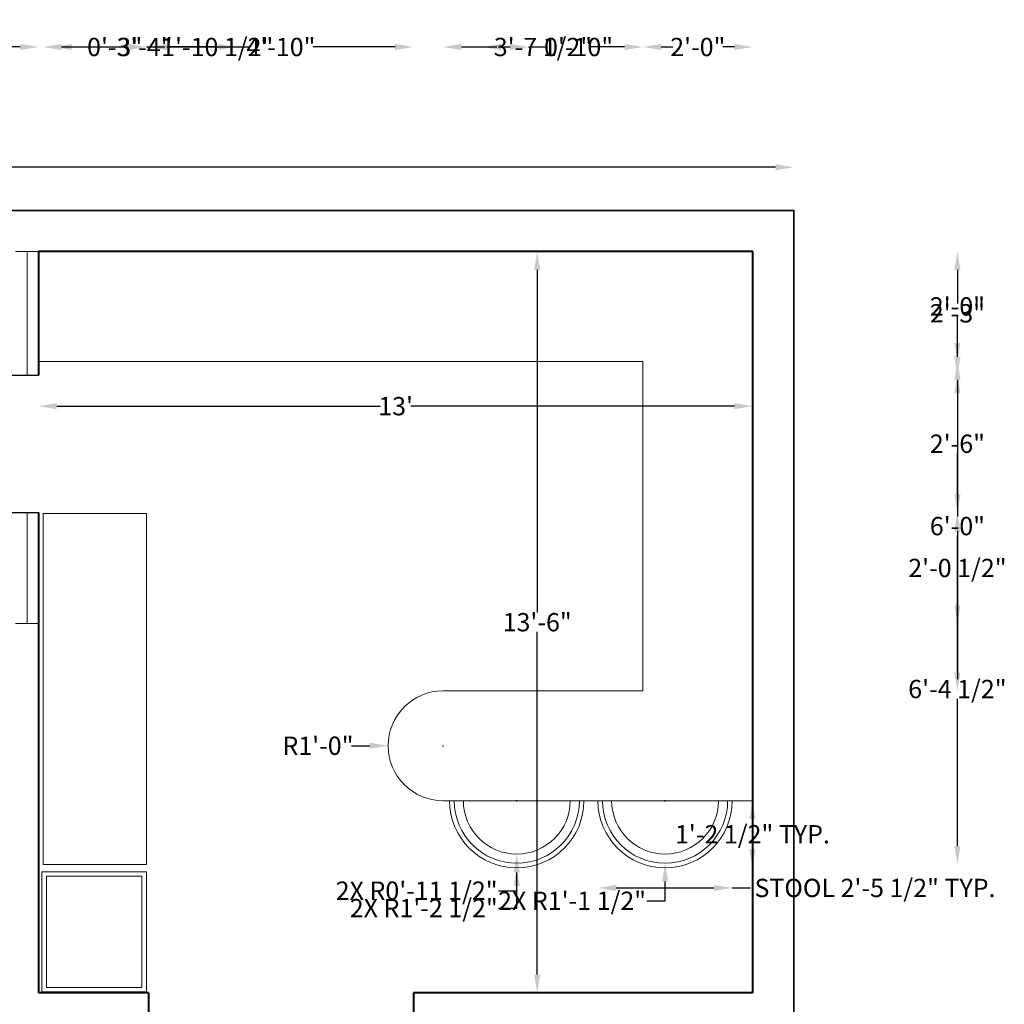
# Model space of a CAD drawing. Units: inches. Extents: x -46 to 447, y -42 to 702.
# Tile 7 of 7: x 227 to 442, y 487 to 702. Entities that reach past the tile are written whole.
import ezdxf

# ---------------------------------------------------------------- set-up
doc = ezdxf.new("R2010")
doc.units = ezdxf.units.IN
doc.header["$PDMODE"] = 3
for name, color, linetype, lineweight in [('A-ANNO-DIMS', 2, 'Continuous', 13), ('A-DOOR', 3, 'Continuous', 25), ('A-FLOR-CASE', 32, 'Continuous', 18), ('A-FURN', 8, 'Continuous', 18), ('A-GLAZ', 4, 'Continuous', 18), ('A-WALL', 7, 'Continuous', 40), ('L-WALL', 7, 'Continuous', 35)]:
    doc.layers.add(name, color=color, linetype=linetype, lineweight=lineweight)
doc.styles.get("Standard").update_dxf_attribs({"font": 'arial.ttf'})
doc.dimstyles.get("Standard").update_dxf_attribs({"dimtxt": 4, "dimasz": 4, "dimexe": 0.18, "dimexo": 0.0625, "dimgap": 0.09, "dimtad": 0, "dimtih": 1, "dimtoh": 1, "dimdec": 0, "dimzin": 0, "dimdsep": 46, "dimlunit": 3, "dimtxsty": 'Standard', "dimcen": 0.09, "dimse1": 1, "dimse2": 1, "dimadec": 0, "dimazin": 0, "dimtfac": 1, "dimtdec": 0, "dimtofl": 0, "dimtmove": 0, "dimatfit": 3, "dimfxl": 1, "dimtolj": 1, "dimtzin": 0, "dimarcsym": 0})

# ---------------------------------------------------------------- blocks, each defined once
blk = doc.blocks.new('*U3')
for p, q in [((-30, 0), (-30, -6)), ((0, 0), (0, -6))]:
    blk.add_line(p, q)
blk.add_lwpolyline([(0, 0), (0, 30), (-1.75, 30), (-1.75, 0)], close=True)
blk.add_arc((0, 0), 30, 90, 180)
blk = doc.blocks.new('*D49')
at = {"layer": 'A-ANNO-DIMS', "color": 0, "lineweight": -2, "transparency": 16777216}
for p, q in [((4, 669.42), (194.52, 669.42)), ((392, 669.42), (201.48, 669.42))]:
    blk.add_line(p, q, dxfattribs=at)
at = {"layer": 'A-ANNO-DIMS', "color": 0, "transparency": 16777216}
for points in [[(4, 670.09), (4, 668.76), (0, 669.42)], [(392, 670.09), (392, 668.76), (396, 669.42)]]:
    blk.add_solid(points, dxfattribs=at)
at = {"layer": 'Defpoints', "color": 0, "transparency": 16777216}
for p in [(396, 669.42), (0, 660), (396, 660)]:
    blk.add_point(p, dxfattribs=at)
at = {"layer": 'A-ANNO-DIMS', "color": 0, "transparency": 16777216, "insert": (198, 669.42), "char_height": 4, "attachment_point": 5}
blk.add_mtext("\\A1;33'", dxfattribs=at)
blk = doc.blocks.new('*D71')
at = {"layer": 'A-ANNO-DIMS', "color": 0, "lineweight": -2, "transparency": 16777216}
for p, q in [((235, 617.21), (305.7, 617.21)), ((383, 617.21), (312.3, 617.21))]:
    blk.add_line(p, q, dxfattribs=at)
at = {"layer": 'A-ANNO-DIMS', "color": 0, "transparency": 16777216}
for points in [[(235, 617.88), (235, 616.55), (231, 617.21)], [(383, 617.88), (383, 616.55), (387, 617.21)]]:
    blk.add_solid(points, dxfattribs=at)
at = {"layer": 'Defpoints', "color": 0, "transparency": 16777216}
for p in [(231, 651), (387, 651), (231, 617.21)]:
    blk.add_point(p, dxfattribs=at)
at = {"layer": 'A-ANNO-DIMS', "color": 0, "transparency": 16777216, "insert": (309, 617.21), "char_height": 4, "attachment_point": 5}
blk.add_mtext("\\A1;13'", dxfattribs=at)
blk = doc.blocks.new('*D72')
at = {"layer": 'A-ANNO-DIMS', "color": 0, "lineweight": -2, "transparency": 16777216}
for p, q in [((339.92, 647), (339.92, 572.13)), ((339.92, 493), (339.92, 567.87))]:
    blk.add_line(p, q, dxfattribs=at)
at = {"layer": 'A-ANNO-DIMS', "color": 0, "transparency": 16777216}
for points in [[(339.26, 647), (340.59, 647), (339.92, 651)], [(339.26, 493), (340.59, 493), (339.92, 489)]]:
    blk.add_solid(points, dxfattribs=at)
at = {"layer": 'Defpoints', "color": 0, "transparency": 16777216}
for p in [(339.92, 651), (387, 651), (387, 489)]:
    blk.add_point(p, dxfattribs=at)
at = {"layer": 'A-ANNO-DIMS', "color": 0, "transparency": 16777216, "insert": (339.92, 570), "char_height": 4, "attachment_point": 5}
blk.add_mtext('\\A1;13\'-6"', dxfattribs=at)
blk = doc.blocks.new('COUNTER-STOOL')
for radius in [14.67, 13.67, 11.67]:
    blk.add_arc((0, 0), radius, 180, 0)
blk = doc.blocks.new('*D102')
at = {"layer": 'A-ANNO-DIMS', "color": 0, "lineweight": -2, "transparency": 16777216}
for p, q in [((357.18, 511.93), (378.53, 511.93)), ((382.53, 511.93), (386.53, 511.93))]:
    blk.add_line(p, q, dxfattribs=at)
at = {"layer": 'A-ANNO-DIMS', "color": 0, "transparency": 16777216}
for points in [[(357.18, 512.59), (357.18, 511.26), (353.18, 511.93)], [(378.53, 512.59), (378.53, 511.26), (382.53, 511.93)]]:
    blk.add_solid(points, dxfattribs=at)
at = {"layer": 'Defpoints', "color": 0, "transparency": 16777216}
for p in [(353.18, 516.33), (382.53, 516.33), (382.53, 511.93)]:
    blk.add_point(p, dxfattribs=at)
at = {"layer": 'A-ANNO-DIMS', "color": 0, "transparency": 16777216, "insert": (413.7, 511.93), "char_height": 4, "attachment_point": 5}
blk.add_mtext('\\A1;STOOL 2\'-5 1/2" TYP.', dxfattribs=at)
blk = doc.blocks.new('*D103')
at = {"layer": 'A-ANNO-DIMS', "color": 0, "lineweight": -2, "transparency": 16777216}
for p, q in [((386.93, 527), (386.93, 525.82)), ((386.93, 520.33), (386.93, 521.51))]:
    blk.add_line(p, q, dxfattribs=at)
at = {"layer": 'A-ANNO-DIMS', "color": 0, "transparency": 16777216}
for points in [[(386.26, 527), (387.59, 527), (386.93, 531)], [(386.26, 520.33), (387.59, 520.33), (386.93, 516.33)]]:
    blk.add_solid(points, dxfattribs=at)
at = {"layer": 'Defpoints', "color": 0, "transparency": 16777216}
for p in [(382.53, 531), (386.93, 531), (382.53, 516.33)]:
    blk.add_point(p, dxfattribs=at)
at = {"layer": 'A-ANNO-DIMS', "color": 0, "transparency": 16777216, "insert": (386.93, 523.66), "char_height": 4, "attachment_point": 5}
blk.add_mtext('\\A1;1\'-2 1/2" TYP.', dxfattribs=at)
blk = doc.blocks.new('*D116')
at = {"layer": 'A-ANNO-DIMS', "color": 0, "lineweight": -2, "transparency": 16777216}
for p, q in [((367, 695.7), (369.56, 695.7)), ((383, 695.7), (380.44, 695.7))]:
    blk.add_line(p, q, dxfattribs=at)
at = {"layer": 'A-ANNO-DIMS', "color": 0, "transparency": 16777216}
for points in [[(367, 696.37), (367, 695.03), (363, 695.7)], [(383, 696.37), (383, 695.03), (387, 695.7)]]:
    blk.add_solid(points, dxfattribs=at)
at = {"layer": 'Defpoints', "color": 0, "transparency": 16777216}
for p in [(387, 695.7), (387, 651), (363, 627)]:
    blk.add_point(p, dxfattribs=at)
at = {"layer": 'A-ANNO-DIMS', "color": 0, "transparency": 16777216, "insert": (375, 695.7), "char_height": 4, "attachment_point": 5}
blk.add_mtext('\\A1;2\'-0"', dxfattribs=at)
blk = doc.blocks.new('*D117')
at = {"layer": 'A-ANNO-DIMS', "color": 0, "lineweight": -2, "transparency": 16777216}
for p, q in [((259, 695.7), (276.91, 695.7)), ((308.89, 695.7), (290.99, 695.7))]:
    blk.add_line(p, q, dxfattribs=at)
at = {"layer": 'A-ANNO-DIMS', "color": 0, "transparency": 16777216}
for points in [[(259, 696.37), (259, 695.03), (255, 695.7)], [(308.89, 696.37), (308.89, 695.03), (312.89, 695.7)]]:
    blk.add_solid(points, dxfattribs=at)
at = {"layer": 'Defpoints', "color": 0, "transparency": 16777216}
for p in [(312.89, 695.7), (255, 489), (312.89, 489)]:
    blk.add_point(p, dxfattribs=at)
at = {"layer": 'A-ANNO-DIMS', "color": 0, "transparency": 16777216, "insert": (283.95, 695.7), "char_height": 4, "attachment_point": 5}
blk.add_mtext('\\A1;4\'-10"', dxfattribs=at)
blk = doc.blocks.new('*D119')
at = {"layer": 'A-ANNO-DIMS', "color": 0, "lineweight": -2, "transparency": 16777216}
for p, q in [((238.24, 695.7), (248.83, 695.7)), ((270.24, 695.7), (259.64, 695.7))]:
    blk.add_line(p, q, dxfattribs=at)
at = {"layer": 'A-ANNO-DIMS', "color": 0, "transparency": 16777216}
for points in [[(238.24, 696.37), (238.24, 695.03), (234.24, 695.7)], [(270.24, 696.37), (270.24, 695.03), (274.24, 695.7)]]:
    blk.add_solid(points, dxfattribs=at)
at = {"layer": 'Defpoints', "color": 0, "transparency": 16777216}
for p in [(274.24, 695.7), (234.24, 319), (274.24, 319)]:
    blk.add_point(p, dxfattribs=at)
at = {"layer": 'A-ANNO-DIMS', "color": 0, "transparency": 16777216, "insert": (254.24, 695.7), "char_height": 4, "attachment_point": 5}
blk.add_mtext('\\A1;3\'-4"', dxfattribs=at)
blk = doc.blocks.new('*D124')
at = {"layer": 'A-ANNO-DIMS', "color": 0, "lineweight": -2, "transparency": 16777216}
for p, q in [((431.7, 620), (431.7, 611.13)), ((431.7, 598), (431.7, 606.87))]:
    blk.add_line(p, q, dxfattribs=at)
at = {"layer": 'A-ANNO-DIMS', "color": 0, "transparency": 16777216}
for points in [[(431.03, 620), (432.37, 620), (431.7, 624)], [(431.03, 598), (432.37, 598), (431.7, 594)]]:
    blk.add_solid(points, dxfattribs=at)
at = {"layer": 'Defpoints', "color": 0, "transparency": 16777216}
for p in [(231, 624), (431.7, 624), (231, 594)]:
    blk.add_point(p, dxfattribs=at)
at = {"layer": 'A-ANNO-DIMS', "color": 0, "transparency": 16777216, "insert": (431.7, 609), "char_height": 4, "attachment_point": 5}
blk.add_mtext('\\A1;2\'-6"', dxfattribs=at)
blk = doc.blocks.new('*D134')
at = {"layer": 'A-ANNO-DIMS', "color": 0, "lineweight": -2, "transparency": 16777216}
for p, q in [((431.7, 623), (431.7, 593.13)), ((431.7, 559), (431.7, 588.87))]:
    blk.add_line(p, q, dxfattribs=at)
at = {"layer": 'A-ANNO-DIMS', "color": 0, "transparency": 16777216}
for points in [[(431.03, 623), (432.37, 623), (431.7, 627)], [(431.03, 559), (432.37, 559), (431.7, 555)]]:
    blk.add_solid(points, dxfattribs=at)
at = {"layer": 'Defpoints', "color": 0, "transparency": 16777216}
for p in [(363, 627), (363, 555), (431.7, 555)]:
    blk.add_point(p, dxfattribs=at)
at = {"layer": 'A-ANNO-DIMS', "color": 0, "transparency": 16777216, "insert": (431.7, 591), "char_height": 4, "attachment_point": 5}
blk.add_mtext('\\A1;6\'-0"', dxfattribs=at)
blk = doc.blocks.new('*D135')
at = {"layer": 'A-ANNO-DIMS', "color": 0, "lineweight": -2, "transparency": 16777216}
for p, q in [((323.36, 695.7), (331.11, 695.7)), ((359, 695.7), (351.25, 695.7))]:
    blk.add_line(p, q, dxfattribs=at)
at = {"layer": 'A-ANNO-DIMS', "color": 0, "transparency": 16777216}
for points in [[(323.36, 696.37), (323.36, 695.03), (319.36, 695.7)], [(359, 696.37), (359, 695.03), (363, 695.7)]]:
    blk.add_solid(points, dxfattribs=at)
at = {"layer": 'Defpoints', "color": 0, "transparency": 16777216}
for p in [(363, 695.7), (319.36, 555), (363, 555)]:
    blk.add_point(p, dxfattribs=at)
at = {"layer": 'A-ANNO-DIMS', "color": 0, "transparency": 16777216, "insert": (341.18, 695.7), "char_height": 4, "attachment_point": 5}
blk.add_mtext('\\A1;3\'-7 1/2"', dxfattribs=at)
blk = doc.blocks.new('*D136')
at = {"layer": 'A-ANNO-DIMS', "color": 0, "lineweight": -2, "transparency": 16777216}
for p, q in [((431.7, 647), (431.7, 641.13)), ((431.7, 631), (431.7, 636.87))]:
    blk.add_line(p, q, dxfattribs=at)
at = {"layer": 'A-ANNO-DIMS', "color": 0, "transparency": 16777216}
for points in [[(431.03, 647), (432.37, 647), (431.7, 651)], [(431.03, 631), (432.37, 631), (431.7, 627)]]:
    blk.add_solid(points, dxfattribs=at)
at = {"layer": 'Defpoints', "color": 0, "transparency": 16777216}
for p in [(387, 651), (431.7, 651), (363, 627)]:
    blk.add_point(p, dxfattribs=at)
at = {"layer": 'A-ANNO-DIMS', "color": 0, "transparency": 16777216, "insert": (431.7, 639), "char_height": 4, "attachment_point": 5}
blk.add_mtext('\\A1;2\'-0"', dxfattribs=at)
blk = doc.blocks.new('*D139')
at = {"layer": 'A-ANNO-DIMS', "color": 0, "lineweight": -2, "transparency": 16777216}
for p, q in [((431.7, 590), (431.7, 584.01)), ((431.7, 573.71), (431.7, 579.7))]:
    blk.add_line(p, q, dxfattribs=at)
at = {"layer": 'A-ANNO-DIMS', "color": 0, "transparency": 16777216}
for points in [[(431.03, 590), (432.37, 590), (431.7, 594)], [(431.03, 573.71), (432.37, 573.71), (431.7, 569.71)]]:
    blk.add_solid(points, dxfattribs=at)
at = {"layer": 'Defpoints', "color": 0, "transparency": 16777216}
for p in [(226, 594), (431.7, 594), (226, 569.71)]:
    blk.add_point(p, dxfattribs=at)
at = {"layer": 'A-ANNO-DIMS', "color": 0, "transparency": 16777216, "insert": (431.7, 581.85), "char_height": 4, "attachment_point": 5}
blk.add_mtext('\\A1;2\'-0 1/2"', dxfattribs=at)
blk = doc.blocks.new('*D142')
at = {"layer": 'A-ANNO-DIMS', "color": 0, "lineweight": -2, "transparency": 16777216}
for p, q in [((431.7, 647), (431.7, 639.63)), ((431.7, 628), (431.7, 635.37))]:
    blk.add_line(p, q, dxfattribs=at)
at = {"layer": 'A-ANNO-DIMS', "color": 0, "transparency": 16777216}
for points in [[(431.03, 647), (432.37, 647), (431.7, 651)], [(431.03, 628), (432.37, 628), (431.7, 624)]]:
    blk.add_solid(points, dxfattribs=at)
at = {"layer": 'Defpoints', "color": 0, "transparency": 16777216}
for p in [(231, 651), (431.7, 651), (231, 624)]:
    blk.add_point(p, dxfattribs=at)
at = {"layer": 'A-ANNO-DIMS', "color": 0, "transparency": 16777216, "insert": (431.7, 637.5), "char_height": 4, "attachment_point": 5}
blk.add_mtext('\\A1;2\'-3"', dxfattribs=at)
blk = doc.blocks.new('*D148')
at = {"layer": 'A-ANNO-DIMS', "color": 0, "lineweight": -2, "transparency": 16777216}
for p, q in [((227, 695.7), (223, 695.7)), ((238.24, 695.7), (242.24, 695.7))]:
    blk.add_line(p, q, dxfattribs=at)
at = {"layer": 'A-ANNO-DIMS', "color": 0, "transparency": 16777216}
for points in [[(227, 696.37), (227, 695.03), (231, 695.7)], [(238.24, 696.37), (238.24, 695.03), (234.24, 695.7)]]:
    blk.add_solid(points, dxfattribs=at)
at = {"layer": 'Defpoints', "color": 0, "transparency": 16777216}
for p in [(234.24, 695.7), (231, 319), (234.24, 319)]:
    blk.add_point(p, dxfattribs=at)
at = {"layer": 'A-ANNO-DIMS', "color": 0, "transparency": 16777216, "insert": (247.64, 695.7), "char_height": 4, "attachment_point": 5}
blk.add_mtext('\\A1;0\'-3"', dxfattribs=at)
blk = doc.blocks.new('*D149')
at = {"layer": 'A-ANNO-DIMS', "color": 0, "lineweight": -2, "transparency": 16777216}
for p, q in [((332, 695.7), (334, 695.7)), ((338, 695.7), (342, 695.7))]:
    blk.add_line(p, q, dxfattribs=at)
at = {"layer": 'A-ANNO-DIMS', "color": 0, "transparency": 16777216}
for points in [[(332, 696.37), (332, 695.03), (328, 695.7)], [(334, 696.37), (334, 695.03), (338, 695.7)]]:
    blk.add_solid(points, dxfattribs=at)
at = {"layer": 'Defpoints', "color": 0, "transparency": 16777216}
for p in [(338, 695.7), (328, 445), (338, 445)]:
    blk.add_point(p, dxfattribs=at)
at = {"layer": 'A-ANNO-DIMS', "color": 0, "transparency": 16777216, "insert": (348.96, 695.7), "char_height": 4, "attachment_point": 5}
blk.add_mtext('\\A1;0\'-10"', dxfattribs=at)
blk = doc.blocks.new('*D151')
at = {"layer": 'A-ANNO-DIMS', "color": 0, "lineweight": -2, "transparency": 16777216}
for p, q in [((236.01, 695.7), (250.6, 695.7)), ((254.6, 695.7), (258.6, 695.7))]:
    blk.add_line(p, q, dxfattribs=at)
at = {"layer": 'A-ANNO-DIMS', "color": 0, "transparency": 16777216}
for points in [[(236.01, 696.37), (236.01, 695.03), (232.01, 695.7)], [(250.6, 696.37), (250.6, 695.03), (254.6, 695.7)]]:
    blk.add_solid(points, dxfattribs=at)
at = {"layer": 'Defpoints', "color": 0, "transparency": 16777216}
for p in [(254.6, 695.7), (232.01, 593.76), (254.6, 593.76)]:
    blk.add_point(p, dxfattribs=at)
at = {"layer": 'A-ANNO-DIMS', "color": 0, "transparency": 16777216, "insert": (270.04, 695.7), "char_height": 4, "attachment_point": 5}
blk.add_mtext('\\A1;1\'-10 1/2"', dxfattribs=at)
blk = doc.blocks.new('*D152')
at = {"layer": 'A-ANNO-DIMS', "color": 0, "lineweight": -2, "transparency": 16777216}
for p, q in [((431.7, 589.76), (431.7, 557.56)), ((431.7, 521.03), (431.7, 553.24))]:
    blk.add_line(p, q, dxfattribs=at)
at = {"layer": 'A-ANNO-DIMS', "color": 0, "transparency": 16777216}
for points in [[(431.03, 589.76), (432.37, 589.76), (431.7, 593.76)], [(431.03, 521.03), (432.37, 521.03), (431.7, 517.03)]]:
    blk.add_solid(points, dxfattribs=at)
at = {"layer": 'Defpoints', "color": 0, "transparency": 16777216}
for p in [(254.6, 593.76), (254.6, 517.03), (431.7, 517.03)]:
    blk.add_point(p, dxfattribs=at)
at = {"layer": 'A-ANNO-DIMS', "color": 0, "transparency": 16777216, "insert": (431.7, 555.4), "char_height": 4, "attachment_point": 5}
blk.add_mtext('\\A1;6\'-4 1/2"', dxfattribs=at)
blk = doc.blocks.new('*D155')
at = {"layer": 'A-ANNO-DIMS', "color": 0, "lineweight": -2, "transparency": 16777216}
for p, q in [((299.36, 543), (303.36, 543)), ((319.27, 543), (319.45, 543)), ((319.36, 542.91), (319.36, 543.09))]:
    blk.add_line(p, q, dxfattribs=at)
at = {"layer": 'A-ANNO-DIMS', "color": 0, "transparency": 16777216}
blk.add_solid([(303.36, 543.67), (303.36, 542.33), (307.36, 543)], dxfattribs=at)
at = {"layer": 'Defpoints', "color": 0, "transparency": 16777216}
for p in [(307.36, 543), (319.36, 543)]:
    blk.add_point(p, dxfattribs=at)
at = {"layer": 'A-ANNO-DIMS', "color": 0, "transparency": 16777216, "insert": (292.04, 543), "char_height": 4, "attachment_point": 5}
blk.add_mtext('\\A1;R1\'-0"', dxfattribs=at)
blk = doc.blocks.new('*D156')
at = {"layer": 'A-ANNO-DIMS', "color": 0, "lineweight": -2, "transparency": 16777216}
for p, q in [((335.37, 531), (335.55, 531)), ((335.46, 530.91), (335.46, 531.09)), ((335.46, 507.52), (335.46, 512.33)), ((331.46, 507.52), (335.46, 507.52))]:
    blk.add_line(p, q, dxfattribs=at)
at = {"layer": 'A-ANNO-DIMS', "color": 0, "transparency": 16777216}
blk.add_solid([(334.79, 512.33), (336.13, 512.33), (335.46, 516.33)], dxfattribs=at)
at = {"layer": 'Defpoints', "color": 0, "transparency": 16777216}
for p in [(335.46, 531), (335.46, 516.33)]:
    blk.add_point(p, dxfattribs=at)
at = {"layer": 'A-ANNO-DIMS', "color": 0, "transparency": 16777216, "insert": (315.15, 507.52), "char_height": 4, "attachment_point": 5}
blk.add_mtext('\\A1;2X R1\'-2 1/2"', dxfattribs=at)
blk = doc.blocks.new('*D157')
at = {"layer": 'A-ANNO-DIMS', "color": 0, "lineweight": -2, "transparency": 16777216}
for p, q in [((367.76, 531), (367.94, 531)), ((367.85, 530.91), (367.85, 531.09)), ((367.85, 509.12), (367.85, 513.33)), ((363.85, 509.12), (367.85, 509.12))]:
    blk.add_line(p, q, dxfattribs=at)
at = {"layer": 'A-ANNO-DIMS', "color": 0, "transparency": 16777216}
blk.add_solid([(367.19, 513.33), (368.52, 513.33), (367.85, 517.33)], dxfattribs=at)
at = {"layer": 'Defpoints', "color": 0, "transparency": 16777216}
for p in [(367.85, 531), (367.85, 517.33)]:
    blk.add_point(p, dxfattribs=at)
at = {"layer": 'A-ANNO-DIMS', "color": 0, "transparency": 16777216, "insert": (347.54, 509.12), "char_height": 4, "attachment_point": 5}
blk.add_mtext('\\A1;2X R1\'-1 1/2"', dxfattribs=at)
blk = doc.blocks.new('*D158')
at = {"layer": 'A-ANNO-DIMS', "color": 0, "lineweight": -2, "transparency": 16777216}
for p, q in [((335.37, 531), (335.55, 531)), ((335.46, 530.91), (335.46, 531.09)), ((335.46, 511.33), (335.46, 515.33)), ((331.46, 511.33), (335.46, 511.33))]:
    blk.add_line(p, q, dxfattribs=at)
at = {"layer": 'A-ANNO-DIMS', "color": 0, "transparency": 16777216}
blk.add_solid([(334.79, 515.33), (336.13, 515.33), (335.46, 519.33)], dxfattribs=at)
at = {"layer": 'Defpoints', "color": 0, "transparency": 16777216}
for p in [(335.46, 531), (335.46, 519.33)]:
    blk.add_point(p, dxfattribs=at)
at = {"layer": 'A-ANNO-DIMS', "color": 0, "transparency": 16777216, "insert": (313.59, 511.33), "char_height": 4, "attachment_point": 5}
blk.add_mtext('\\A1;2X R0\'-11 1/2"', dxfattribs=at)

msp = doc.modelspace()

# ---------------------------------------------------------------- linework, layer by layer
at = {"layer": 'A-FLOR-CASE'}
for p, q in [((231, 627), (363, 627)), ((363, 555), (363, 627)), ((363, 555), (319.36, 555)), ((319.36, 531), (387, 531))]:
    msp.add_line(p, q, dxfattribs=at)
for points in [[(254.6, 517.03), (232.01, 517.03), (232.01, 593.76), (254.6, 593.76)], [(254.6, 489.19), (231.76, 489.19), (231.76, 515.47), (254.6, 515.47)], [(253.6, 490.19), (232.76, 490.19), (232.76, 514.47), (253.6, 514.47)]]:
    msp.add_lwpolyline(points, close=True, dxfattribs=at)
msp.add_arc((319.36, 543), 12, 90, 270, dxfattribs=at)
at = {"layer": 'A-GLAZ'}
for p, q in [((226, 651), (231, 651)), ((228.5, 651), (228.5, 624)), ((231, 624), (226, 624)), ((228.5, 569.71), (228.5, 594)), ((226, 569.71), (231, 569.71))]:
    msp.add_line(p, q, dxfattribs=at)
at = {"layer": 'A-WALL'}
for p, q in [((387, 651), (231, 651)), ((231, 651), (231, 624)), ((387, 489), (387, 651)), ((231, 594), (231, 489)), ((255, 489), (231, 489)), ((255, 489), (255, 484)), ((387, 489), (312.89, 489)), ((312.89, 489), (312.89, 484))]:
    msp.add_line(p, q, dxfattribs=at)
at = {"layer": 'L-WALL'}
msp.add_lwpolyline([(222, 0), (396, 0), (396, 660), (0, 660), (0, 0), (17.93, 0)], dxfattribs=at)

# ---------------------------------------------------------------- block references
at = {"layer": 'A-DOOR', "xscale": -1, "rotation": 90}
msp.add_blockref('*U3', (225, 594), dxfattribs=at)
at = {"layer": 'A-FURN'}
for p in [(335.46, 531), (367.85, 531)]:
    msp.add_blockref('COUNTER-STOOL', p, dxfattribs=at)

# ---------------------------------------------------------------- dimensions: what is measured, and where the dimension line sits
at = {"layer": 'A-ANNO-DIMS'}
for base, p1, p2, override, picture, middle in [((254.6, 695.7), (232.01, 593.76), (254.6, 593.76), {"dimdec": 1, "dimlfac": 1, "dimrnd": 0, "dimzin": 1, "dimdsep": 46, "dimlunit": 4, "dimfrac": 2}, '*D151', (270.04, 695.7)), ((363, 695.7), (319.36, 555), (363, 555), {"dimdec": 1, "dimlfac": 1, "dimrnd": 0, "dimzin": 1, "dimdsep": 46, "dimlunit": 4, "dimfrac": 2}, '*D135', (341.18, 695.7)), ((234.24, 695.7), (231, 319), (234.24, 319), {"dimdec": 1, "dimlfac": 1, "dimrnd": 0, "dimzin": 1, "dimdsep": 46, "dimlunit": 4, "dimfrac": 2}, '*D148', (247.64, 695.7)), ((274.24, 695.7), (234.24, 319), (274.24, 319), {"dimdec": 1, "dimlfac": 1, "dimrnd": 0, "dimzin": 1, "dimdsep": 46, "dimlunit": 4, "dimfrac": 2}, '*D119', (254.24, 695.7)), ((312.89, 695.7), (255, 489), (312.89, 489), {"dimdec": 1, "dimlfac": 1, "dimrnd": 0, "dimzin": 1, "dimdsep": 46, "dimlunit": 4, "dimfrac": 2}, '*D117', (283.95, 695.7)), ((338, 695.7), (328, 445), (338, 445), {"dimdec": 1, "dimlfac": 1, "dimrnd": 0, "dimzin": 1, "dimdsep": 46, "dimlunit": 4, "dimfrac": 2}, '*D149', (348.96, 695.7)), ((387, 695.7), (363, 627), (387, 651), {"dimdec": 1, "dimlfac": 1, "dimrnd": 0, "dimzin": 1, "dimdsep": 46, "dimlunit": 4, "dimfrac": 2}, '*D116', (375, 695.7)), ((396, 669.42), (0, 660), (396, 660), {"dimclrd": 0, "dimclre": 0, "dimclrt": 0}, '*D49', (198, 669.42)), ((231, 617.21), (387, 651), (231, 651), {"dimclrd": 0, "dimclre": 0, "dimclrt": 0}, '*D71', (309, 617.21))]:
    dim = msp.add_linear_dim(base=base, p1=p1, p2=p2, dimstyle='Standard', override=override, dxfattribs=at)
    dim.commit()
    dim.dimension.update_dxf_attribs({"geometry": picture, "text_midpoint": middle})
for base, p1, p2, override, picture, middle in [((431.7, 651), (231, 624), (231, 651), {"dimdec": 1, "dimlfac": 1, "dimrnd": 0, "dimzin": 1, "dimdsep": 46, "dimlunit": 4, "dimfrac": 2}, '*D142', (431.7, 637.5)), ((339.92, 651), (387, 489), (387, 651), {"dimclrd": 0, "dimclre": 0, "dimclrt": 0}, '*D72', (339.92, 570)), ((431.7, 651), (363, 627), (387, 651), {"dimdec": 1, "dimlfac": 1, "dimrnd": 0, "dimzin": 1, "dimdsep": 46, "dimlunit": 4, "dimfrac": 2}, '*D136', (431.7, 639)), ((431.7, 555), (363, 627), (363, 555), {"dimdec": 1, "dimlfac": 1, "dimrnd": 0, "dimzin": 1, "dimdsep": 46, "dimlunit": 4, "dimfrac": 2}, '*D134', (431.7, 591)), ((431.7, 624), (231, 594), (231, 624), {"dimdec": 1, "dimlfac": 1, "dimrnd": 0, "dimzin": 1, "dimdsep": 46, "dimlunit": 4, "dimfrac": 2}, '*D124', (431.7, 609)), ((431.7, 594), (226, 569.71), (226, 594), {"dimdec": 1, "dimlfac": 1, "dimrnd": 0, "dimzin": 1, "dimdsep": 46, "dimlunit": 4, "dimfrac": 2}, '*D139', (431.7, 581.85)), ((431.7, 517.03), (254.6, 593.76), (254.6, 517.03), {"dimdec": 1, "dimlfac": 1, "dimrnd": 0, "dimzin": 1, "dimdsep": 46, "dimlunit": 4, "dimfrac": 2}, '*D152', (431.7, 555.4))]:
    dim = msp.add_linear_dim(base=base, p1=p1, p2=p2, angle=90, dimstyle='Standard', override=override, dxfattribs=at)
    dim.commit()
    dim.dimension.update_dxf_attribs({"geometry": picture, "text_midpoint": middle})
dim = msp.add_radius_dim(center=(319.36, 543), mpoint=(307.36, 543), dimstyle='Standard', override={"dimdec": 1, "dimlfac": 1, "dimrnd": 0, "dimzin": 1, "dimdsep": 46, "dimlunit": 4, "dimfrac": 2}, dxfattribs=at)
dim.commit()
dim.dimension.update_dxf_attribs({"geometry": '*D155', "text_midpoint": (292.04, 543)})
dim = msp.add_linear_dim(base=(386.93, 531), p1=(382.53, 516.33), p2=(382.53, 531), angle=90, text='<> TYP.', dimstyle='Standard', override={"dimdec": 1, "dimlfac": 1, "dimrnd": 0, "dimzin": 1, "dimdsep": 46, "dimlunit": 4, "dimfrac": 2}, dxfattribs=at)
dim.commit()
dim.dimension.update_dxf_attribs({"geometry": '*D103', "text_midpoint": (386.93, 523.66)})
dim = msp.add_radius_dim(center=(335.46, 531), mpoint=(335.46, 519.33), text='2X <>', dimstyle='Standard', override={"dimdec": 1, "dimlfac": 1, "dimrnd": 0, "dimzin": 1, "dimdsep": 46, "dimlunit": 4, "dimfrac": 2}, dxfattribs=at)
dim.commit()
dim.dimension.update_dxf_attribs({"geometry": '*D158', "text_midpoint": (313.59, 511.33)})
for center, mpoint, picture, middle in [((335.46, 531), (335.46, 516.33), '*D156', (315.15, 507.52)), ((367.85, 531), (367.85, 517.33), '*D157', (347.54, 509.12))]:
    dim = msp.add_radius_dim(center=center, mpoint=mpoint, text='2X <>', dimstyle='Standard', override={"dimdec": 1, "dimlfac": 1, "dimrnd": 0, "dimzin": 1, "dimdsep": 46, "dimlunit": 4, "dimfrac": 2}, dxfattribs=at)
    dim.commit()
    dim.dimension.update_dxf_attribs({"geometry": picture, "text_midpoint": middle, "dimtype": 164})
dim = msp.add_linear_dim(base=(382.5263, 511.925), p1=(353.1802, 516.3269), p2=(382.5263, 516.3269), text='STOOL <> TYP.', dimstyle='Standard', override={"dimdec": 1, "dimlfac": 1, "dimrnd": 0, "dimzin": 1, "dimdsep": 46, "dimlunit": 4, "dimfrac": 2}, dxfattribs=at)
dim.commit()
dim.dimension.update_dxf_attribs({"geometry": '*D102', "text_midpoint": (413.705, 511.925)})

doc.saveas('drawing.dxf')
